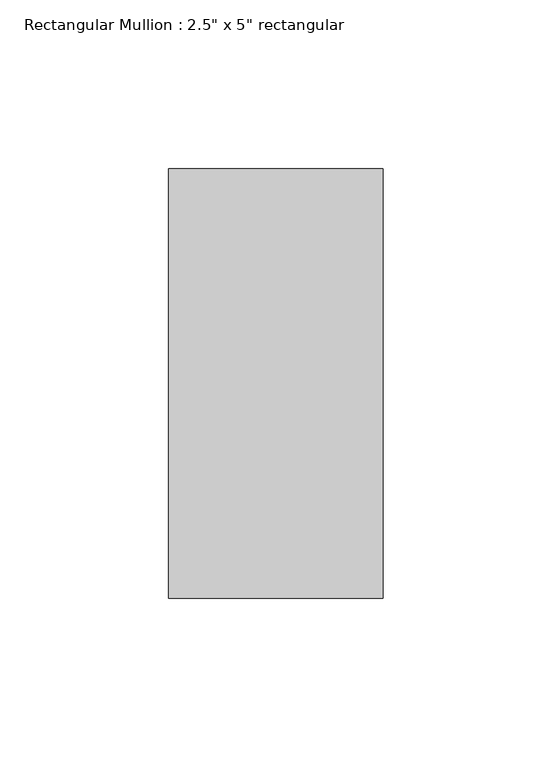
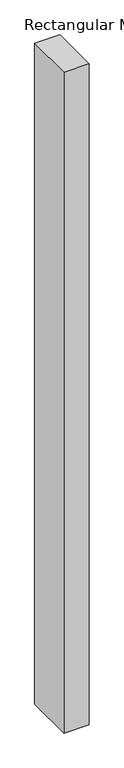
"""IFC4 building model written with IfcOpenShell, lengths in millimetres: member geometry."""

from ifc_helpers import new_model, si_unit, frame, origin, place, context, project, spatial, polyline, outline, extrude, source, transform, mapped, element, save


def member_de80672f(model_context):
    return source(origin(), model_context, "Body", "SweptSolid", [
        extrude(outline(polyline([(31.75, 63.5), (31.75, -63.5), (-31.75, -63.5), (-31.75, 63.5), (31.75, 63.5)])), frame((0.0, 0.0, -1757.093674), z_axis=(0.0, 0.0, 1.0), x_axis=(1.0, 0.0, 0.0)), (0.0, 0.0, 1.0), 1757.093674),
    ])


if __name__ == "__main__":
    model = new_model("IFC4")
    model_context = context("Model", 3, world=origin())
    ifc_project = project(units=[si_unit("LENGTHUNIT", "METRE", prefix="MILLI")], contexts=[model_context])
    site = spatial("IfcSite", under=ifc_project)
    building = spatial("IfcBuilding", under=site)
    placement = place(None, origin())
    member_shape = member_de80672f(model_context)
    element("IfcMember", 1, ObjectType="Rectangular Mullion : 2.5\" x 5\" rectangular", at=placement, inside=building, context=model_context, shape_type="MappedRepresentation", body=[
        mapped(member_shape, transform((0.0, 0.0, 0.0), x_axis=(1.0, 0.0, 0.0), y_axis=(0.0, 1.0, 0.0), z_axis=(0.0, 0.0, 1.0))),
    ])
    save(model, "model.ifc")

# Revit data of these elements
# Type "Rectangular Mullion : 2.5\" x 5\" rectangular"
#   built-in parameter 1007304 = 0.416667 (stored number, unit not read)
#   built-in parameter 1007301 = 0.104167 (stored number, unit not read)
#   built-in parameter 1007300 = 0.104167 (stored number, unit not read)
# Element 1 (IfcMember, "Rectangular Mullion : 2.5\" x 5\" rectangular")
#   Materials on its faces: "Aluminum"
# Materials
#   "Aluminum": class "Metal", colour RGB 247 247 247, transparency 0, Description = "Aluminum 6061", Cost = 0
